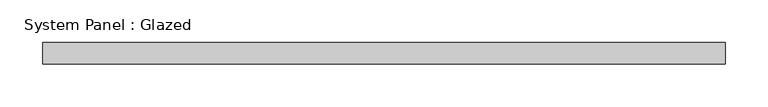
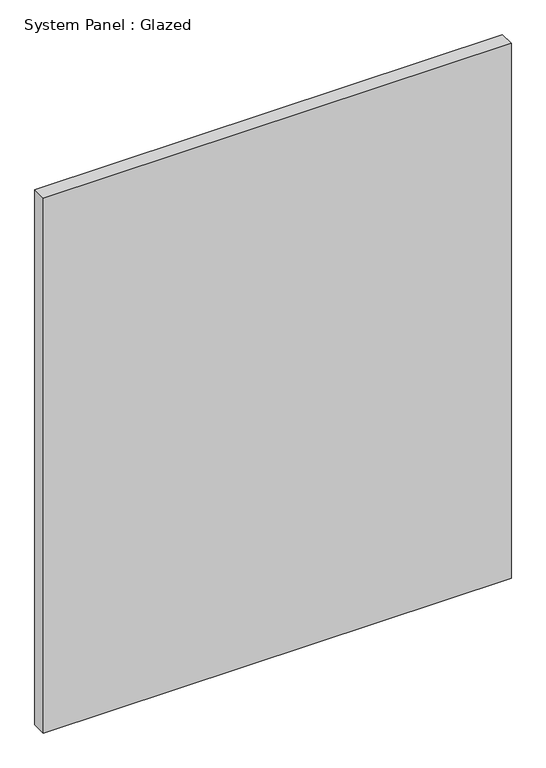
"""IFC4 building model written with IfcOpenShell, lengths in millimetres: plate geometry, System Panel : Glazed."""

from ifc_helpers import new_model, si_unit, origin, origin_with_axes, place, context, project, spatial, polyline, outline, extrude, source, transform, mapped, element, save


def system_panel_glazed_52a3cc88(model_context):
    return source(origin(), model_context, "Body", "SweptSolid", [
        extrude(outline(polyline([(399.6200545, 19.05), (-399.6200545, 19.05), (-399.6200545, 44.45), (399.6200545, 44.45), (399.6200545, 19.05)])), origin_with_axes(), (0.0, 0.0, 1.0), 965.2),
    ])


if __name__ == "__main__":
    model = new_model("IFC4")
    model_context = context("Model", 3, world=origin())
    ifc_project = project(units=[si_unit("LENGTHUNIT", "METRE", prefix="MILLI")], contexts=[model_context])
    site = spatial("IfcSite", under=ifc_project)
    building = spatial("IfcBuilding", under=site)
    placement = place(None, origin())
    system_panel_glazed_shape = system_panel_glazed_52a3cc88(model_context)
    element("IfcPlate", 1, ObjectType="System Panel : Glazed", at=placement, inside=building, context=model_context, shape_type="MappedRepresentation", body=[
        mapped(system_panel_glazed_shape, transform((0.0, 0.0, 0.0), x_axis=(1.0, 0.0, 0.0), y_axis=(0.0, 1.0, 0.0), z_axis=(0.0, 0.0, 1.0))),
    ])
    save(model, "model.ifc")

# Revit data of these elements
# Type "System Panel : Glazed"
#   Construction Type Id = "GSP4R"
#   Analytic Construction = "1/8 in Pilkington single glazing"
#   Visual Light Transmittance = 0.9
#   Solar Heat Gain Coefficient = 0.86
#   Heat Transfer Coefficient (U) = 1.18115 BTU/(h·ft²·°F)
# Element 1 (IfcPlate, "System Panel : Glazed")
#   Materials on its faces: "Glass"
# Materials
#   "Glass": class "Glass", colour RGB 0 128 192, transparency 0.75, Description = "Soda Lime Glass", Cost = 0
